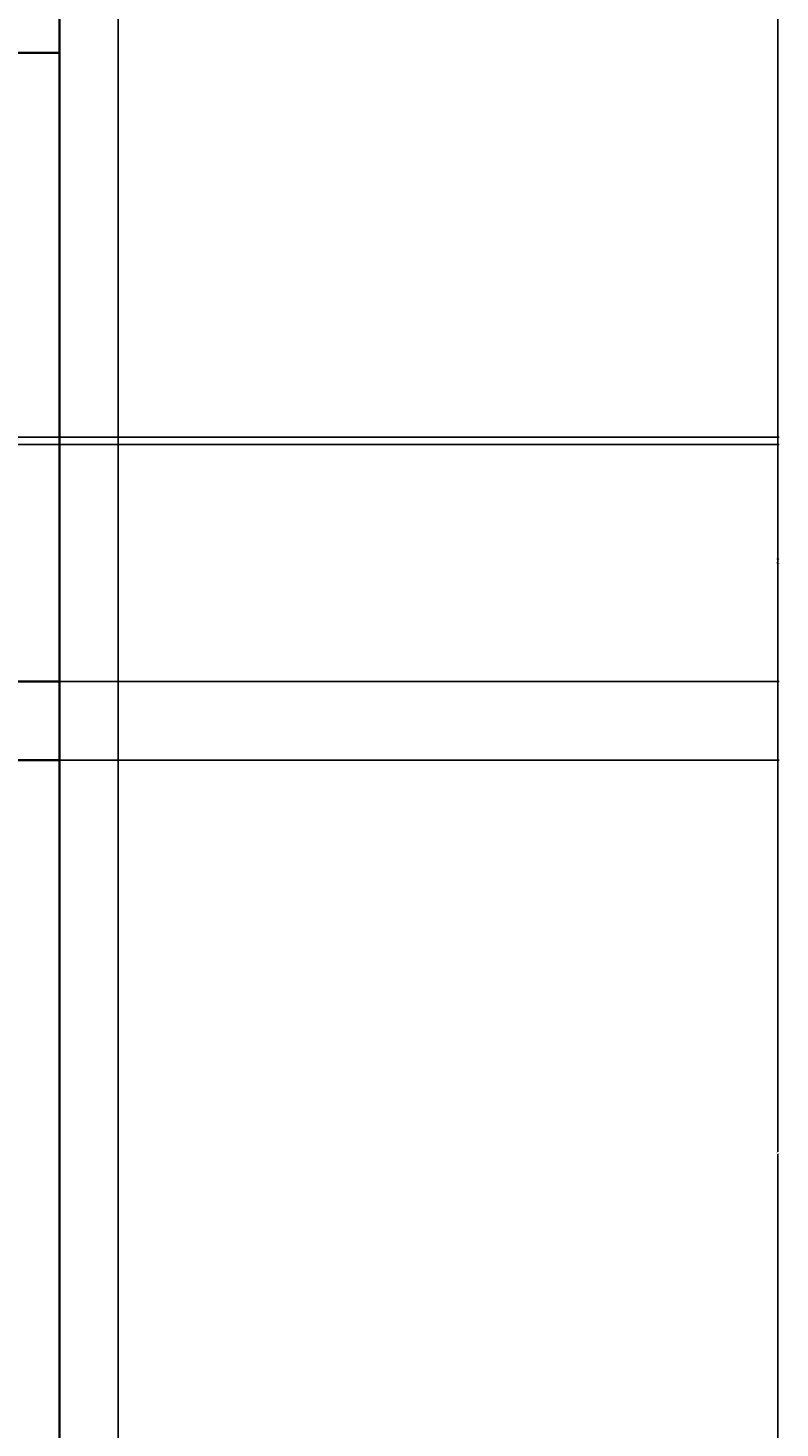
# Model space of a CAD drawing. Units: inches. Extents: x -8 to 554, y -200 to 499.
# Tile 11 of 12: x 440 to 554, y 121 to 335. Entities that reach past the tile are written whole.
import ezdxf

# ---------------------------------------------------------------- set-up
doc = ezdxf.new("R2010")
doc.units = ezdxf.units.IN
doc.header["$MEASUREMENT"] = 0
for name, color, linetype, lineweight in [('A-ANNO-DIMS', 2, 'Continuous', 18), ('A-FLOR', 7, 'Continuous', 35), ('A-WALL', 7, 'Continuous', 35), ('A-WALL-PRPT', 7, 'Continuous', 25)]:
    doc.layers.add(name, color=color, linetype=linetype, lineweight=lineweight)
doc.styles.get("Standard").update_dxf_attribs({"font": 'arial.ttf'})
doc.dimstyles.get("Standard").update_dxf_attribs({"dimtxt": 0.18, "dimasz": 0.18, "dimexe": 0.18, "dimexo": 0.0625, "dimgap": 0.09, "dimtad": 0, "dimtih": 1, "dimtoh": 1, "dimdec": 4, "dimzin": 0, "dimdsep": 46, "dimtxsty": 'Standard', "dimcen": 0.09, "dimadec": 0, "dimazin": 0, "dimtfac": 1, "dimtdec": 4, "dimtofl": 0, "dimtmove": 0, "dimatfit": 3, "dimfxl": 1, "dimtolj": 1, "dimtzin": 0, "dimarcsym": 0})

# ---------------------------------------------------------------- blocks, each defined once
blk = doc.blocks.new('*D30')
at = {"layer": 'A-ANNO-DIMS', "color": 0, "lineweight": -2, "transparency": 16777216}
for p, q in [((444.4, 439.48), (554.26, 439.48)), ((554.08, 439.3), (554.08, 163.66)), ((554.08, -112.34), (554.08, 163.3)), ((446.15, -112.52), (554.26, -112.52))]:
    blk.add_line(p, q, dxfattribs=at)
at = {"layer": 'A-ANNO-DIMS', "color": 0, "transparency": 16777216}
for points in [[(554.05, 439.3), (554.11, 439.3), (554.08, 439.48)], [(554.05, -112.34), (554.11, -112.34), (554.08, -112.52)]]:
    blk.add_solid(points, dxfattribs=at)
at = {"layer": 'Defpoints', "color": 0, "transparency": 16777216}
for p in [(444.34, 439.48), (446.09, -112.52), (554.08, -112.52)]:
    blk.add_point(p, dxfattribs=at)
at = {"layer": 'A-ANNO-DIMS', "color": 0, "transparency": 16777216, "insert": (554.08, 163.48), "char_height": 0.18, "attachment_point": 5}
blk.add_mtext('\\A1;552', dxfattribs=at)
blk = doc.blocks.new('*D31')
at = {"layer": 'A-ANNO-DIMS', "color": 0, "lineweight": -2, "transparency": 16777216}
for p, q in [((24.34, 127.42), (24.34, -199.97)), ((453.32, -30.73), (453.32, -199.97)), ((24.52, -199.79), (238.54, -199.79)), ((453.14, -199.79), (239.12, -199.79))]:
    blk.add_line(p, q, dxfattribs=at)
at = {"layer": 'A-ANNO-DIMS', "color": 0, "transparency": 16777216}
for points in [[(24.52, -199.76), (24.52, -199.82), (24.34, -199.79)], [(453.14, -199.76), (453.14, -199.82), (453.32, -199.79)]]:
    blk.add_solid(points, dxfattribs=at)
at = {"layer": 'Defpoints', "color": 0, "transparency": 16777216}
for p in [(24.34, 127.48), (453.32, -30.67), (453.32, -199.79)]:
    blk.add_point(p, dxfattribs=at)
at = {"layer": 'A-ANNO-DIMS', "color": 0, "transparency": 16777216, "insert": (238.83, -199.79), "char_height": 0.18, "attachment_point": 5}
blk.add_mtext('\\A1;429', dxfattribs=at)
blk = doc.blocks.new('*D32')
at = {"layer": 'A-ANNO-DIMS', "color": 0, "lineweight": -2, "transparency": 16777216}
for p, q in [((24.34, 223.42), (24.34, -199.97)), ((444.34, 223.42), (444.34, -199.97)), ((24.52, -199.79), (234.05, -199.79)), ((444.16, -199.79), (234.63, -199.79))]:
    blk.add_line(p, q, dxfattribs=at)
at = {"layer": 'A-ANNO-DIMS', "color": 0, "transparency": 16777216}
for points in [[(24.52, -199.76), (24.52, -199.82), (24.34, -199.79)], [(444.16, -199.76), (444.16, -199.82), (444.34, -199.79)]]:
    blk.add_solid(points, dxfattribs=at)
at = {"layer": 'Defpoints', "color": 0, "transparency": 16777216}
for p in [(24.34, 223.48), (444.34, 223.48), (444.34, -199.79)]:
    blk.add_point(p, dxfattribs=at)
at = {"layer": 'A-ANNO-DIMS', "color": 0, "transparency": 16777216, "insert": (234.34, -199.79), "char_height": 0.18, "attachment_point": 5}
blk.add_mtext('\\A1;420', dxfattribs=at)
blk = doc.blocks.new('*D38')
at = {"layer": 'A-ANNO-DIMS', "color": 0, "lineweight": -2, "transparency": 16777216}
for p, q in [((444.4, 235.48), (554.26, 235.48)), ((554.08, 235.3), (554.08, 229.66)), ((554.08, 223.66), (554.08, 229.3)), ((444.4, 223.48), (554.26, 223.48))]:
    blk.add_line(p, q, dxfattribs=at)
at = {"layer": 'A-ANNO-DIMS', "color": 0, "transparency": 16777216}
for points in [[(554.05, 235.3), (554.11, 235.3), (554.08, 235.48)], [(554.05, 223.66), (554.11, 223.66), (554.08, 223.48)]]:
    blk.add_solid(points, dxfattribs=at)
at = {"layer": 'Defpoints', "color": 0, "transparency": 16777216}
for p in [(444.34, 235.48), (554.08, 235.48), (444.34, 223.48)]:
    blk.add_point(p, dxfattribs=at)
at = {"layer": 'A-ANNO-DIMS', "color": 0, "transparency": 16777216, "insert": (554.08, 229.48), "char_height": 0.18, "attachment_point": 5}
blk.add_mtext('\\A1;12', dxfattribs=at)
blk = doc.blocks.new('*D46')
at = {"layer": 'A-ANNO-DIMS', "color": 0, "lineweight": -2, "transparency": 16777216}
for p, q in [((101.04, 271.66), (554.26, 271.66)), ((554.08, 271.48), (554.08, 253.75)), ((554.08, 235.66), (554.08, 253.39)), ((66.27, 235.48), (554.26, 235.48))]:
    blk.add_line(p, q, dxfattribs=at)
at = {"layer": 'A-ANNO-DIMS', "color": 0, "transparency": 16777216}
for points in [[(554.05, 271.48), (554.11, 271.48), (554.08, 271.66)], [(554.05, 235.66), (554.11, 235.66), (554.08, 235.48)]]:
    blk.add_solid(points, dxfattribs=at)
at = {"layer": 'Defpoints', "color": 0, "transparency": 16777216}
for p in [(100.98, 271.66), (66.2, 235.48), (554.08, 235.48)]:
    blk.add_point(p, dxfattribs=at)
at = {"layer": 'A-ANNO-DIMS', "color": 0, "transparency": 16777216, "insert": (554.08, 253.57), "char_height": 0.18, "attachment_point": 5}
blk.add_mtext('\\A1;36.18', dxfattribs=at)
blk = doc.blocks.new('*D47')
at = {"layer": 'A-ANNO-DIMS', "color": 0, "lineweight": -2, "transparency": 16777216}
for p, q in [((357.76, 272.76), (554.26, 272.76)), ((554.08, 272.58), (554.08, 254.3)), ((554.08, 235.66), (554.08, 253.94)), ((312.4, 235.48), (554.26, 235.48))]:
    blk.add_line(p, q, dxfattribs=at)
at = {"layer": 'A-ANNO-DIMS', "color": 0, "transparency": 16777216}
for points in [[(554.05, 272.58), (554.11, 272.58), (554.08, 272.76)], [(554.05, 235.66), (554.11, 235.66), (554.08, 235.48)]]:
    blk.add_solid(points, dxfattribs=at)
at = {"layer": 'Defpoints', "color": 0, "transparency": 16777216}
for p in [(357.7, 272.76), (312.34, 235.48), (554.08, 235.48)]:
    blk.add_point(p, dxfattribs=at)
at = {"layer": 'A-ANNO-DIMS', "color": 0, "transparency": 16777216, "insert": (554.08, 254.12), "char_height": 0.18, "attachment_point": 5}
blk.add_mtext('\\A1;37.28', dxfattribs=at)
blk = doc.blocks.new('*D55')
at = {"layer": 'A-ANNO-DIMS', "color": 0, "lineweight": -2, "transparency": 16777216}
for p, q in [((204.61, -30.61), (204.61, 498.99)), ((204.79, 498.81), (328.57, 498.81)), ((453.14, 498.81), (329.36, 498.81)), ((453.32, -30.61), (453.32, 498.99))]:
    blk.add_line(p, q, dxfattribs=at)
at = {"layer": 'A-ANNO-DIMS', "color": 0, "transparency": 16777216}
for points in [[(204.79, 498.84), (204.79, 498.78), (204.61, 498.81)], [(453.14, 498.84), (453.14, 498.78), (453.32, 498.81)]]:
    blk.add_solid(points, dxfattribs=at)
at = {"layer": 'Defpoints', "color": 0, "transparency": 16777216}
for p in [(453.32, 498.81), (204.61, -30.67), (453.32, -30.67)]:
    blk.add_point(p, dxfattribs=at)
at = {"layer": 'A-ANNO-DIMS', "color": 0, "transparency": 16777216, "insert": (328.96, 498.81), "char_height": 0.18, "attachment_point": 5}
blk.add_mtext('\\A1;248.7', dxfattribs=at)
blk = doc.blocks.new('*D71')
at = {"layer": 'A-ANNO-DIMS', "color": 0, "lineweight": -2, "transparency": 16777216}
for p, q in [((444.34, 439.42), (444.34, -199.97)), ((432.52, 427.42), (432.52, -199.97)), ((432.7, -199.79), (437.97, -199.79)), ((444.16, -199.79), (438.89, -199.79))]:
    blk.add_line(p, q, dxfattribs=at)
at = {"layer": 'A-ANNO-DIMS', "color": 0, "transparency": 16777216}
for points in [[(432.7, -199.76), (432.7, -199.82), (432.52, -199.79)], [(444.16, -199.76), (444.16, -199.82), (444.34, -199.79)]]:
    blk.add_solid(points, dxfattribs=at)
at = {"layer": 'Defpoints', "color": 0, "transparency": 16777216}
for p in [(444.34, 439.48), (432.52, 427.48), (444.34, -199.79)]:
    blk.add_point(p, dxfattribs=at)
at = {"layer": 'A-ANNO-DIMS', "color": 0, "transparency": 16777216, "insert": (438.43, -199.79), "char_height": 0.18, "attachment_point": 5}
blk.add_mtext('\\A1;11.825', dxfattribs=at)

msp = doc.modelspace()

# ---------------------------------------------------------------- linework, layer by layer
at = {"layer": 'A-FLOR'}
for p, q in [((444.3421, 331.4814), (36.3421, 331.4814)), ((444.3421, 235.4814), (24.3421, 235.4814)), ((36.3421, 235.4814), (444.3421, 235.4814)), ((24.3421, 223.4814), (444.3421, 223.4814)), ((444.3421, 223.4814), (36.3421, 223.4814))]:
    msp.add_line(p, q, dxfattribs=at)
at = {"layer": 'A-WALL'}
for p, q in [((444.3421, 223.4814), (444.3421, 343.4814)), ((444.3421, 115.4814), (444.3421, 235.4814)), ((444.3421, 7.4814), (444.3421, 127.4814))]:
    msp.add_line(p, q, dxfattribs=at)
at = {"layer": 'A-WALL-PRPT'}
for points in [[(444.3421, 155.7921), (444.3421, 127.4814)], [(444.3421, 147.4508), (444.3421, 148.5204)], [(444.3421, 141.4657), (444.3421, 142.5354)], [(444.3421, 135.7657), (444.3421, 136.8354)]]:
    msp.add_lwpolyline(points, dxfattribs=at)

# ---------------------------------------------------------------- dimensions: what is measured, and where the dimension line sits
at = {"layer": 'A-ANNO-DIMS'}
for base, p1, p2, override, picture, middle in [((453.3222, 498.8091), (204.6055, -30.6677), (453.3222, -30.6677), {"dimdec": 1, "dimlfac": 1, "dimrnd": 0, "dimzin": 0, "dimdsep": 46, "dimlunit": 2}, '*D55', (328.9639, 498.8091)), ((444.3421, -199.7912), (432.5174, 427.4814), (444.3421, 439.4814), {"dimdec": 3, "dimlfac": 1, "dimrnd": 0, "dimzin": 0, "dimdsep": 46, "dimlunit": 2}, '*D71', (438.4297, -199.7912)), ((444.3421, -199.7912), (24.3421, 223.4814), (444.3421, 223.4814), {"dimdec": 0, "dimlfac": 1, "dimrnd": 0, "dimzin": 0, "dimdsep": 46, "dimlunit": 2}, '*D32', (234.3421, -199.7912)), ((453.3222, -199.7912), (24.3421, 127.4814), (453.3222, -30.6677), {"dimdec": 0, "dimlfac": 1, "dimrnd": 0, "dimzin": 0, "dimdsep": 46, "dimlunit": 2}, '*D31', (238.8321, -199.7912))]:
    dim = msp.add_linear_dim(base=base, p1=p1, p2=p2, dimstyle='Standard', override=override, dxfattribs=at)
    dim.commit()
    dim.dimension.update_dxf_attribs({"geometry": picture, "text_midpoint": middle})
for base, p1, p2, override, picture, middle in [((554.0833, -112.5186), (444.3421, 439.4814), (446.0855, -112.5186), {"dimdec": 0, "dimlfac": 1, "dimrnd": 0, "dimzin": 0, "dimdsep": 46, "dimlunit": 2}, '*D30', (554.0833, 163.4814)), ((554.0833, 235.4814), (100.9765, 271.661), (66.2048, 235.4814), {"dimdec": 2, "dimlfac": 1, "dimrnd": 0, "dimzin": 0, "dimdsep": 46, "dimlunit": 2}, '*D46', (554.0833, 253.5712)), ((554.0833, 235.4814), (357.699, 272.7623), (312.3421, 235.4814), {"dimdec": 2, "dimlfac": 1, "dimrnd": 0, "dimzin": 0, "dimdsep": 46, "dimlunit": 2}, '*D47', (554.0833, 254.1218)), ((554.0833, 235.4814), (444.3421, 223.4814), (444.3421, 235.4814), {"dimdec": 0, "dimlfac": 1, "dimrnd": 0, "dimzin": 0, "dimdsep": 46, "dimlunit": 2}, '*D38', (554.0833, 229.4814))]:
    dim = msp.add_linear_dim(base=base, p1=p1, p2=p2, angle=90, dimstyle='Standard', override=override, dxfattribs=at)
    dim.commit()
    dim.dimension.update_dxf_attribs({"geometry": picture, "text_midpoint": middle})

doc.saveas('drawing.dxf')
